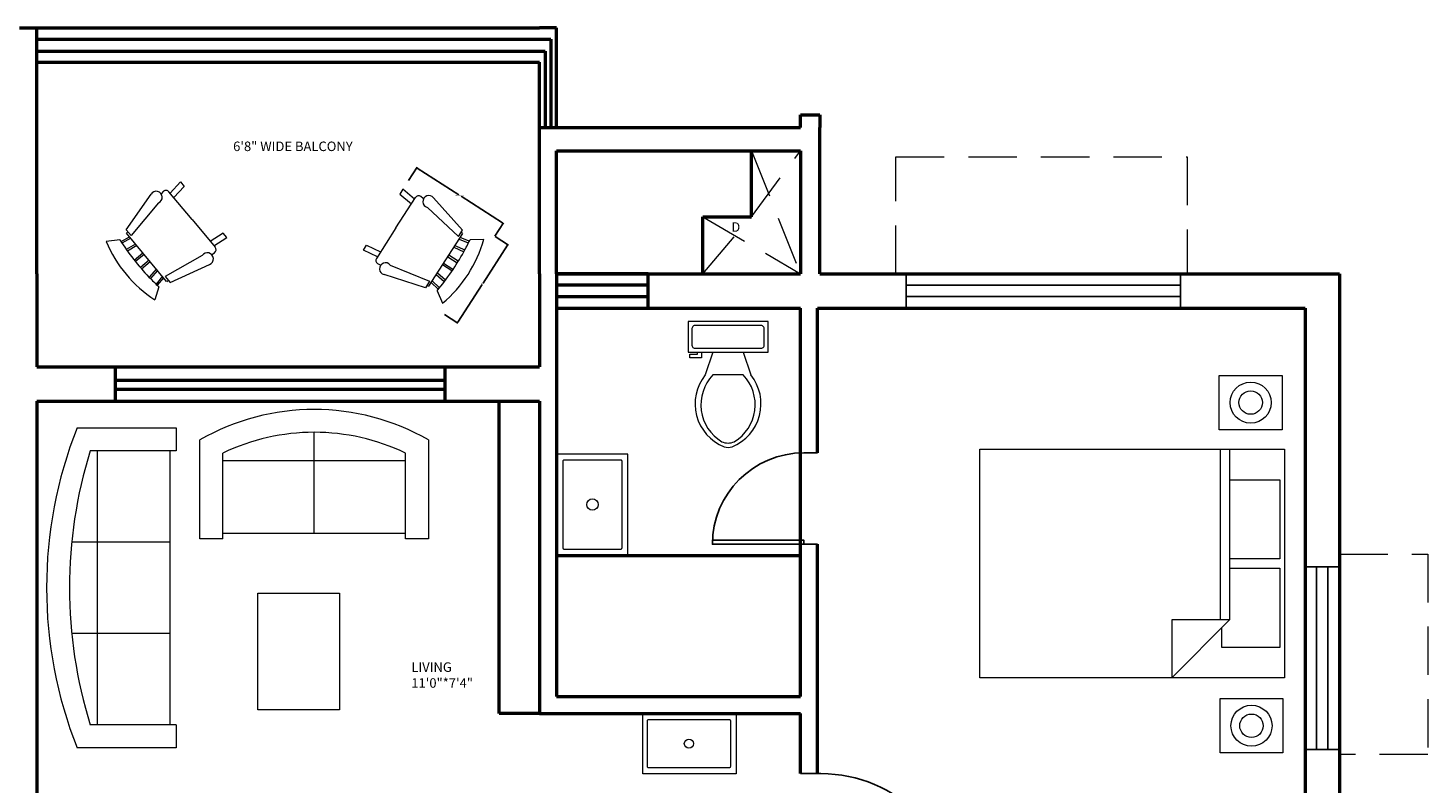
# Model space of a CAD drawing. Units: inches. Extents: x 291 to 2631, y 456 to 2623.
# Tile 22 of 22: x 2205 to 2572, y 2425 to 2623. Entities that reach past the tile are written whole.
import ezdxf

# ---------------------------------------------------------------- set-up
doc = ezdxf.new("R2010")
doc.units = ezdxf.units.IN
doc.linetypes.add('DASHED', pattern=[19.05, 12.7, -6.35])
for name, color, linetype, lineweight in [('A-ANNO-DIMS', 2, 'Continuous', 18), ('A-ANNO-TEXT', 3, 'Continuous', 25), ('A-AREA-IDEN', 7, 'Continuous', 25), ('A-DOOR', 3, 'Continuous', 25), ('A-FLOR-FIXT', 9, 'Continuous', 18), ('A-FLOR-OVHD', 1, 'DASHED', 18), ('A-FURN', 8, 'Continuous', 18), ('A-GLAZ', 4, 'Continuous', 25), ('A-WALL', 7, 'Continuous', 50)]:
    doc.layers.add(name, color=color, linetype=linetype, lineweight=lineweight)
doc.styles.get("Standard").update_dxf_attribs({"font": 'arial.ttf'})
doc.dimstyles.get("Standard").update_dxf_attribs({"dimtxt": 0.18, "dimasz": 0.18, "dimexe": 0.18, "dimexo": 0.0625, "dimgap": 0.09, "dimtad": 0, "dimtih": 1, "dimtoh": 1, "dimdec": 4, "dimzin": 0, "dimdsep": 46, "dimtxsty": 'Standard', "dimcen": 0.09, "dimadec": 0, "dimazin": 0, "dimtfac": 1, "dimtdec": 4, "dimtofl": 0, "dimtmove": 0, "dimatfit": 3, "dimfxl": 1, "dimtolj": 1, "dimtzin": 0, "dimarcsym": 0})

# ---------------------------------------------------------------- blocks, each defined once
blk = doc.blocks.new('*U2')
for p, q in [((0, 0), (0, -6)), ((40, 0), (40, -6))]:
    blk.add_line(p, q)
blk.add_lwpolyline([(0, 0), (0, 40), (1.75, 40), (1.75, 0)], close=True)
blk.add_arc((0, 0), 40, 0, 90)
blk = doc.blocks.new('Bed - Queen')
for p, q in [((0, -80.00003), (0, 0)), ((0, 0), (59.99999, 0)), ((59.99999, 0), (59.99999, -80.00003)), ((7.99999, -1.2), (28.79998, -1.2)), ((7.99999, -14.4), (7.99999, -1.2)), ((28.79998, -1.2), (28.79998, -14.4)), ((31.19999, -1.2), (51.99999, -1.2)), ((31.19999, -14.4), (31.19999, -1.2)), ((51.99999, -1.2), (51.99999, -16.4)), ((0, -14.4), (44.8, -14.4)), ((59.99999, -29.6), (44.8, -14.4)), ((44.8, -14.4), (44.8, -29.6)), ((44.8, -16.8), (0, -16.8)), ((51.99999, -16.4), (46.79936, -16.4)), ((44.8, -29.6), (59.99999, -29.6)), ((59.99999, -80.00003), (0, -80.00003))]:
    blk.add_line(p, q)
blk = doc.blocks.new('Chair - Rocking')
for p, q in [((-8, -4.5), (-10, -1.5)), ((8, -4.5), (10, -1.5)), ((-8.23428, -6.99939), (-8.3093, -7.47958)), ((-8.23041, -7), (8.23915, -7)), ((-7.5, -4.5), (-7, -7)), ((-6.5, -7), (-7.02225, -4.43)), ((-4.5, -7), (-4.96674, -4.19951)), ((-4, -7), (-4.40532, -4.16272)), ((-1.5, -4.05012), (-1.5, -7)), ((-1, -7), (-1, -4.05012)), ((1, -7), (1, -4.04655)), ((1.5, -4.05012), (1.5, -7)), ((4, -7), (4.40187, -4.18694)), ((4.5, -7), (4.96761, -4.19437)), ((6.5, -7), (7, -4.4057)), ((7.5, -4.5), (7, -7)), ((8.31071, -7.48854), (8.23449, -7.00073)), ((-9, -7.5), (-12, -18.49999)), ((-7, -7.5), (-9, -7.5)), ((-9, -18.49999), (-7, -7.5)), ((7, -7.5), (9, -7.5)), ((9, -18.49999), (7, -7.5)), ((9, -7.5), (12, -18.49999)), ((-10.36644, -20.64523), (-10.5, -21.49999)), ((10.5, -21.49999), (10.3575, -20.58798)), ((-9, -22.49999), (-9.5, -26.49999)), ((0, -22.49999), (-9.5, -22.49999)), ((-8, -26.49999), (-7.5, -22.49999)), ((0, -22.49999), (9.5, -22.49999)), ((8, -26.49999), (7.5, -22.49999)), ((9, -22.49999), (9.5, -26.49999)), ((-9.5, -26.49999), (-8, -26.49999)), ((9.5, -26.49999), (8, -26.49999))]:
    blk.add_line(p, q)
for centre, radius, start, end in [((0, -34.08333), 34.08333, 72.93847, 107.0615), ((0, -68.25004), 64.25, 93.92211, 97.15267), ((0, -68.25004), 64.25, 82.84733, 93.92211), ((-10.5, -18.99999), 1.58114, 161.5651, 18.43495), ((-9.5, -21.49999), 1, 180, 270), ((10.5, -18.99999), 1.58114, 161.5651, 18.43495), ((9.5, -21.49999), 1, 270, 0)]:
    blk.add_arc(centre, radius, start, end)
blk = doc.blocks.new('Toilet - top')
for p, q in [((9.5, -6), (9.5, -2)), ((-10, -8.5), (-8, -8.5)), ((-10, -9.5), (-10, -8.5)), ((-7, -9.5), (-10, -9.5)), ((-8, -8.5), (-8, -8)), ((-7, -8), (-7, -9.5)), ((-4, -8), (-6, -14)), ((4, -8), (6, -14)), ((4, -14), (-4, -14))]:
    blk.add_line(p, q)
blk.add_lwpolyline([(10.5, -8), (10.5, 0), (-10.5, 0), (-10.5, -8)], close=True)
for points in [[(-9.5, -2), (-9.5, -6)], [(8.5, -1), (-8.5, -1)], [(-8.5, -7), (8.5, -7)]]:
    blk.add_lwpolyline(points)
for centre, radius, start, end in [((-8.62, -1.88), 0.884, 81.8699, 188.1301), ((8.62, -1.88), 0.884, 351.8699, 98.1301), ((-8.62, -6.12), 0.884, 171.8699, 278.1301), ((8.62, -6.12), 0.884, 261.8699, 8.1301), ((3.52, -21.58), 12.17, 141.4691, 247.9714), ((4.2, -21.82), 11.33, 136.3677, 238.9468), ((-3.52, -21.58), 12.17, 292.0284, 38.5307), ((-4.2, -21.82), 11.33, 301.053, 43.6321), ((0, -27.88), 4, 245.7318, 294.2682), ((0, -29), 4, 254.8605, 285.1395)]:
    blk.add_arc(centre, radius, start, end)
blk = doc.blocks.new('Sofa - Roundback 7 ft.')
for p, q in [((-12.00002, -32.4421), (-12.00003, -6.5971)), ((11.99997, -32.4421), (11.99998, -6.5971)), ((-36.000027, -34), (-36.000027, -11.4696)), ((-35.999844, -13.3819), (35.9998, -13.3819)), ((35.99998, -34), (35.99998, -11.4696)), ((-36.000027, -32.4421), (35.99998, -32.4421))]:
    blk.add_line(p, q)
for points in [[(-36.000027, -34), (-42.000027, -34), (-42.000027, -8)], [(41.99998, -8), (41.99998, -34), (35.99998, -34)]]:
    blk.add_lwpolyline(points)
for centre, radius, start, end in [((0, -114.25), 114.25, 68.43141, 111.5686), ((-0.00001, -127.1968), 121.1968, 72.72033, 107.2797)]:
    blk.add_arc(centre, radius, start, end)
blk = doc.blocks.new('Sofa - Roundback Loveseat 5 ft.')
for p, q in [((0, -32.44198), (0, -5.99998)), ((-24, -33.99998), (-24, -11.46958)), ((-23.9998, -13.38178), (23.99986, -13.38178)), ((24.00004, -33.99998), (24.00004, -11.46958)), ((-24, -32.44198), (24.00004, -32.44198))]:
    blk.add_line(p, q)
for points in [[(-24, -33.99998), (-30, -33.99998), (-30, -7.99998)], [(30.00004, -7.99998), (30.00004, -33.99998), (24.00004, -33.99998)]]:
    blk.add_lwpolyline(points)
for centre, radius, start, end in [((0, -60.24998), 60.24998, 60.13715, 119.8628), ((0, -61.38438), 55.38444, 64.32083, 115.6792)]:
    blk.add_arc(centre, radius, start, end)
blk = doc.blocks.new('WIN-1800')
for p, q in [((0, 9), (72, 9)), ((0, 0), (0, 9)), ((72, 9), (72, 0)), ((0, 6), (72, 6)), ((72, 3), (0, 3)), ((72, 0), (0, 0))]:
    blk.add_line(p, q)
blk = doc.blocks.new('WIN-1200')
for p, q in [((0, 0), (0, 48)), ((0, 48), (9, 48)), ((3, 0), (3, 48)), ((6, 48), (6, 0)), ((9, 48), (9, 0)), ((9, 0), (0, 0))]:
    blk.add_line(p, q)
blk = doc.blocks.new('*D32')
at = {"layer": 'A-ANNO-DIMS', "color": 0, "lineweight": -2, "transparency": 16777216}
for p, q in [((2304.6, 2583.25), (2306.86, 2586.75)), ((2306.91, 2586.5), (2317.82, 2579.47)), ((2329.3, 2572.07), (2318.39, 2579.1)), ((2327.29, 2568.62), (2329.55, 2572.12))]:
    blk.add_line(p, q, dxfattribs=at)
at = {"layer": 'A-ANNO-DIMS', "color": 0, "transparency": 16777216}
for points in [[(2306.93, 2586.53), (2306.9, 2586.48), (2306.76, 2586.6)], [(2329.32, 2572.09), (2329.29, 2572.04), (2329.45, 2571.97)]]:
    blk.add_solid(points, dxfattribs=at)
at = {"layer": 'DEFPOINTS', "color": 0, "transparency": 16777216}
for p in [(2304.57, 2583.2), (2329.45, 2571.97), (2327.26, 2568.57)]:
    blk.add_point(p, dxfattribs=at)
at = {"layer": 'A-ANNO-DIMS', "color": 0, "transparency": 16777216, "insert": (2318.11, 2579.28), "char_height": 0.18, "attachment_point": 5}
blk.add_mtext('\\A1;ROCKING CHAIR 27 TYP.', dxfattribs=at)
blk = doc.blocks.new('*D33')
at = {"layer": 'A-ANNO-DIMS', "color": 0, "lineweight": -2, "transparency": 16777216}
for p, q in [((2330.57, 2566.22), (2324.16, 2556.28)), ((2327.31, 2568.53), (2330.82, 2566.27)), ((2317.52, 2545.99), (2323.93, 2555.92)), ((2314.07, 2548), (2317.57, 2545.74))]:
    blk.add_line(p, q, dxfattribs=at)
at = {"layer": 'A-ANNO-DIMS', "color": 0, "transparency": 16777216}
for points in [[(2330.54, 2566.24), (2330.59, 2566.2), (2330.66, 2566.37)], [(2317.5, 2546), (2317.55, 2545.97), (2317.42, 2545.83)]]:
    blk.add_solid(points, dxfattribs=at)
at = {"layer": 'DEFPOINTS', "color": 0, "transparency": 16777216}
for p in [(2327.26, 2568.57), (2314.02, 2548.03), (2317.42, 2545.83)]:
    blk.add_point(p, dxfattribs=at)
at = {"layer": 'A-ANNO-DIMS', "color": 0, "transparency": 16777216, "insert": (2324.04, 2556.1), "char_height": 0.18, "attachment_point": 5}
blk.add_mtext('\\A1;24 TYP.', dxfattribs=at)

msp = doc.modelspace()

# ---------------------------------------------------------------- linework, layer by layer
at = {"layer": 'A-FLOR-OVHD'}
for p, q in [((2394.63, 2591), (2407.49, 2558.74)), ((2394.63, 2573.72), (2407.49, 2591)), ((2432.54, 2558.74), (2432.54, 2589.44)), ((2432.54, 2589.44), (2509.02, 2589.44)), ((2509.02, 2589.44), (2509.02, 2558.74)), ((2381.86, 2573.72), (2407.49, 2558.74)), ((2381.86, 2558.74), (2394.63, 2573.72)), ((2548.99, 2485.14), (2572.25, 2485.14)), ((2572.25, 2485.14), (2572.25, 2432.47)), ((2572.25, 2432.47), (2548.99, 2432.47))]:
    msp.add_line(p, q, dxfattribs=at)
at = {"layer": 'A-FURN'}
for points in [[(2517.46, 2532.06), (2533.94, 2532.06), (2533.94, 2517.76), (2517.46, 2517.76)], [(2343.49, 2484.74), (2362.18, 2484.74), (2362.18, 2511.35), (2343.49, 2511.35)], [(2265.02, 2474.89), (2286.45, 2474.89), (2286.45, 2444.26), (2265.02, 2444.26)], [(2517.67, 2447.21), (2534.15, 2447.21), (2534.15, 2432.91), (2517.67, 2432.91)], [(2366.12, 2443.24), (2390.66, 2443.24), (2390.66, 2427.45), (2366.12, 2427.45)]]:
    msp.add_lwpolyline(points, close=True, dxfattribs=at)
for points in [[(2345.4, 2486.46), (2360.36, 2486.46, 0.414214), (2360.66, 2486.76), (2360.66, 2509.5, 0.414214), (2360.36, 2509.8), (2345.4, 2509.8, 0.414214), (2345.1, 2509.5), (2345.1, 2486.76, 0.414214)], [(2367.65, 2441.7), (2388.79, 2441.7, -0.414214), (2389.09, 2441.4), (2389.09, 2429.32, -0.414214), (2388.79, 2429.02), (2367.65, 2429.02, -0.414214), (2367.35, 2429.32), (2367.35, 2441.4, -0.414214)]]:
    msp.add_lwpolyline(points, format="xyb", close=True, dxfattribs=at)
for centre, radius in [((2525.7, 2524.91), 5.39), ((2525.7, 2524.91), 3.08), ((2352.88, 2498.13), 1.5), ((2525.91, 2440.06), 5.39), ((2525.91, 2440.06), 3.08), ((2378.22, 2435.36), 1.21)]:
    msp.add_circle(centre, radius, dxfattribs=at)
at = {"layer": 'A-WALL'}
for p, q in [((2202.49, 2623.27), (2206.99, 2623.27)), ((2206.99, 2623.27), (2338.99, 2623.27)), ((2206.99, 2558.74), (2206.99, 2623.27)), ((2343.49, 2623.27), (2338.99, 2623.27)), ((2343.49, 2597.17), (2343.49, 2623.27)), ((2206.99, 2620.35), (2338.99, 2620.35)), ((2206.99, 2617.17), (2338.99, 2617.17)), ((2338.99, 2620.35), (2341.97, 2620.35)), ((2338.99, 2617.17), (2340.46, 2617.17)), ((2340.46, 2617.17), (2340.46, 2597.17)), ((2341.97, 2620.35), (2341.97, 2597.17)), ((2206.99, 2614.27), (2338.99, 2614.27)), ((2338.99, 2558.74), (2338.99, 2614.27)), ((2407.49, 2597.17), (2407.49, 2600.48)), ((2407.49, 2600.48), (2412.6, 2600.48)), ((2412.6, 2600.48), (2412.6, 2597.17)), ((2338.99, 2597.17), (2407.49, 2597.17)), ((2412.6, 2558.74), (2412.6, 2597.17)), ((2343.49, 2558.74), (2343.49, 2591)), ((2343.49, 2591), (2407.49, 2591)), ((2394.63, 2573.72), (2394.63, 2591)), ((2407.49, 2591), (2407.49, 2558.74)), ((2381.86, 2558.74), (2381.86, 2573.72)), ((2381.86, 2573.72), (2394.63, 2573.72)), ((2206.99, 2558.74), (2206.99, 2534.27)), ((2338.99, 2558.74), (2338.99, 2534.27)), ((2343.49, 2558.74), (2343.49, 2549.74)), ((2343.49, 2558.74), (2407.49, 2558.74)), ((2367.49, 2558.74), (2343.49, 2558.74)), ((2343.49, 2558.74), (2343.49, 2549.74)), ((2367.49, 2549.74), (2367.49, 2558.74)), ((2412.6, 2558.74), (2548.99, 2558.74)), ((2548.99, 2558.74), (2548.99, 2156.24)), ((2367.49, 2555.74), (2343.49, 2555.74)), ((2343.49, 2552.74), (2367.49, 2552.74)), ((2343.49, 2549.74), (2407.49, 2549.74)), ((2343.49, 2549.74), (2343.49, 2447.74)), ((2343.49, 2549.74), (2367.49, 2549.74)), ((2407.49, 2447.74), (2407.49, 2549.74)), ((2411.99, 2511.72), (2411.99, 2549.74)), ((2411.99, 2549.74), (2539.99, 2549.74)), ((2412.6, 2549.69), (2412.6, 2549.74)), ((2539.99, 2549.74), (2539.99, 2389.74)), ((2206.99, 2534.27), (2338.99, 2534.27)), ((2227.58, 2534.27), (2227.58, 2525.27)), ((2314.13, 2534.27), (2314.13, 2525.27)), ((2227.58, 2530.78), (2314.13, 2530.78)), ((2206.99, 2525.27), (2338.99, 2525.27)), ((2206.99, 2525.27), (2206.99, 2400.18)), ((2227.58, 2528.4), (2314.13, 2528.4)), ((2328.43, 2443.24), (2328.43, 2525.27)), ((2338.99, 2525.27), (2338.99, 2443.24)), ((2343.49, 2484.74), (2407.49, 2484.74)), ((2411.99, 2427.48), (2411.99, 2487.72)), ((2343.49, 2447.74), (2407.49, 2447.74)), ((2338.99, 2443.24), (2328.43, 2443.24)), ((2338.99, 2443.24), (2407.49, 2443.24)), ((2407.49, 2427.48), (2407.49, 2443.24))]:
    msp.add_line(p, q, dxfattribs=at)

# ---------------------------------------------------------------- block references
at = {"layer": 'A-DOOR'}
for p, xscale, yscale, zscale, rotation in [((2408.39, 2487.72), 0.6, 0.6, 0.6, 90.00000000000003), ((2412.89, 2391.48), -0.9, 0.9, 0.9, 270)]:
    msp.add_blockref('*U2', p, dxfattribs=dict(at, xscale=xscale, yscale=yscale, zscale=zscale, rotation=rotation))
at = {"layer": 'A-FLOR-FIXT'}
msp.add_blockref('Toilet - top', (2388.49, 2546.16), dxfattribs=at)
at = {"layer": 'A-FURN'}
for name, p, rotation in [('Chair - Rocking', (2230.46, 2558.59), 129.7567937851614), ('Chair - Rocking', (2320.22, 2558.57), 237.1884930017563), ('Sofa - Roundback 7 ft.', (2209.58, 2476.27), 90), ('Bed - Queen', (2534.56, 2512.64), 270)]:
    msp.add_blockref(name, p, dxfattribs=dict(at, rotation=rotation))
msp.add_blockref('Sofa - Roundback Loveseat 5 ft.', (2279.83, 2523.1), dxfattribs=at)
at = {"layer": 'A-GLAZ'}
for name, p in [('WIN-1800', (2435.26, 2549.74)), ('WIN-1200', (2539.99, 2433.8))]:
    msp.add_blockref(name, p, dxfattribs=at)

# ---------------------------------------------------------------- texts
at = {"layer": 'A-ANNO-TEXT', "insert": (2389.35, 2572.25), "char_height": 2.5, "attachment_point": 1}
msp.add_mtext_dynamic_manual_height_columns('D', width=1.3143, gutter_width=12.5, heights=[0], dxfattribs=at)
at = {"layer": 'A-AREA-IDEN', "char_height": 2.5, "attachment_point": 1}
for s, width, insert in [('6\'8" WIDE BALCONY', 62.0841, (2258.56, 2593.45)), ('LIVING\\P11\'0"*7\'4"', 29.0209, (2305.34, 2456.7))]:
    msp.add_mtext_dynamic_manual_height_columns(s, width=width, gutter_width=12.5, heights=[0], dxfattribs=dict(at, insert=insert))

# ---------------------------------------------------------------- dimensions: what is measured, and where the dimension line sits
at = {"layer": 'A-ANNO-DIMS'}
for base, p1, p2, angle, text, picture, middle in [((2329.45, 2571.97), (2304.57, 2583.2), (2327.26, 2568.57), 327.1885, 'ROCKING CHAIR <> TYP.', '*D32', (2318.11, 2579.28)), ((2317.42, 2545.83), (2327.26, 2568.57), (2314.02, 2548.03), 237.1885, '<> TYP.', '*D33', (2324.04, 2556.1))]:
    dim = msp.add_linear_dim(base=base, p1=p1, p2=p2, angle=angle, text=text, dimstyle='Standard', override={"dimdec": 0, "dimlfac": 1, "dimrnd": 0, "dimzin": 0, "dimdsep": 46, "dimlunit": 2}, dxfattribs=at)
    dim.commit()
    dim.dimension.update_dxf_attribs({"geometry": picture, "text_midpoint": middle})

doc.saveas('drawing.dxf')
